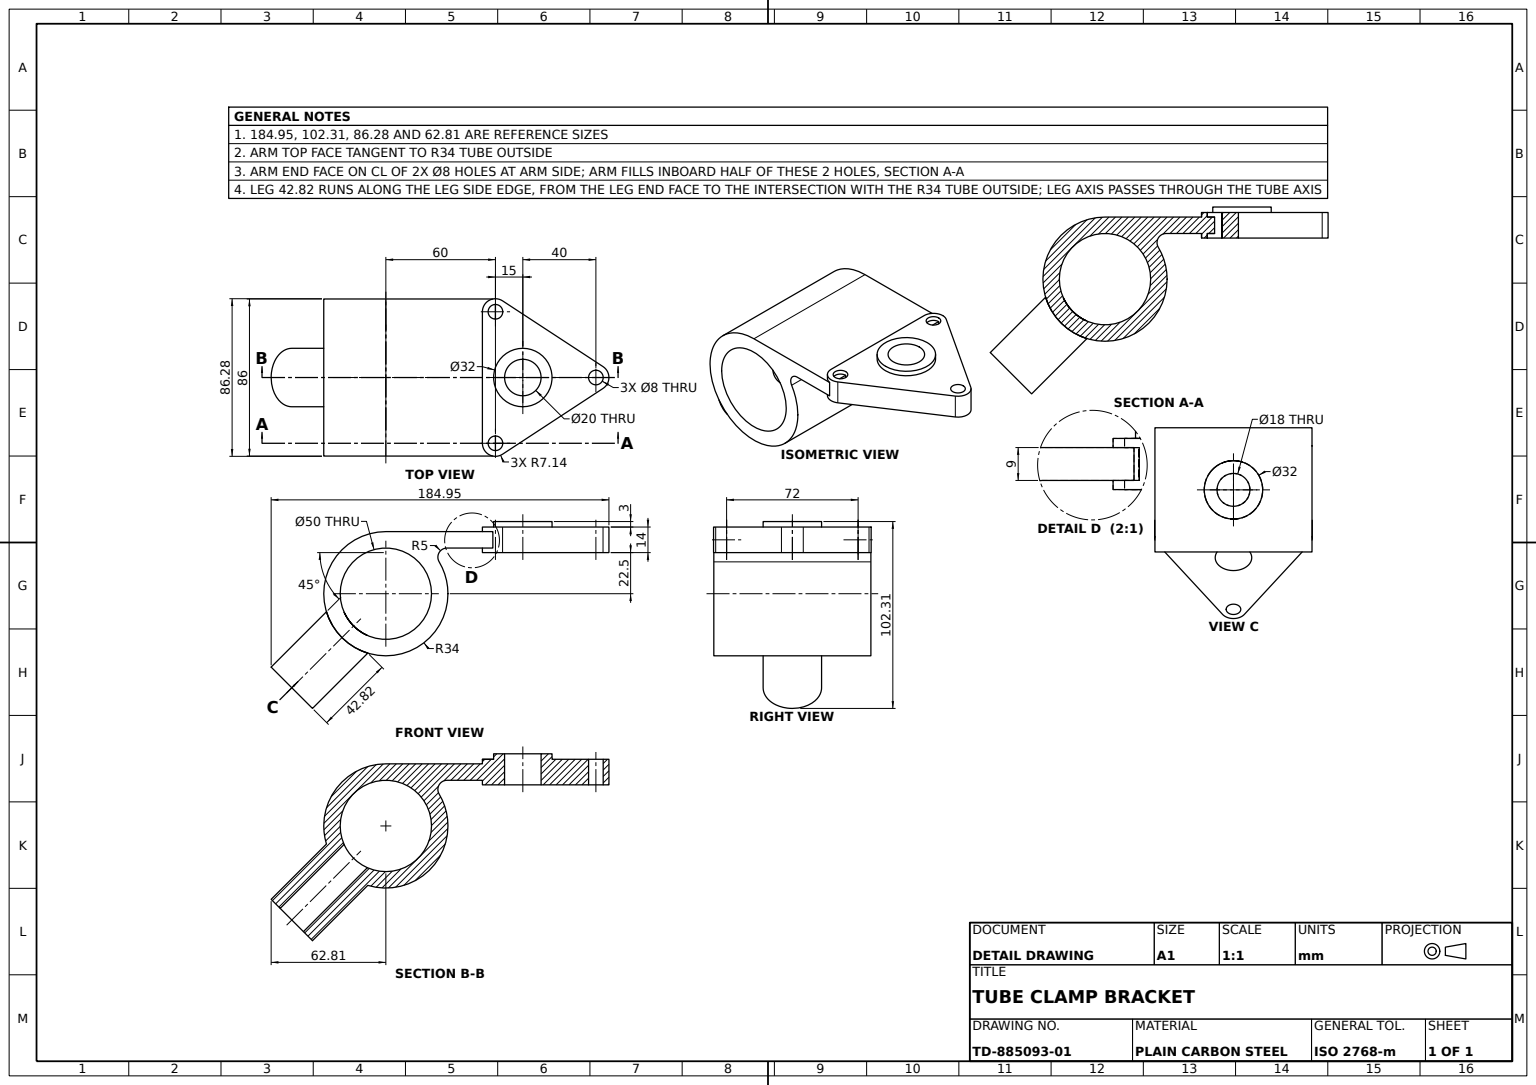
from build123d import *

# Parameters (mm, degrees)
RING_HUB_PROFILE_R       = 25
RING_HUB_DEPTH           = 43
FLANGE_PROFILE_3_HOLES_R = 4
TRIANGULAR_FLANGE_DEPTH  = 7
BOSS_BORE_PROFILE_R      = 10
BOSS_BORE_DEPTH          = 13
FLANGE_START             = 3
FLANGE_BOSS_PROFILE_R    = 16
FLANGE_BOSS_PROFILE_R_2  = 10
FLANGE_BOSS_32_DEPTH     = 3
HUB_SLIT_PROFILE_R       = 9
HUB_SLIT_CUT_DEPTH       = 67.5


with BuildPart() as part:
    # Ring Hub Profile → Ring Hub (new, symmetric)
    with BuildSketch(Plane.XY):
        with BuildLine():
            Line((0, 34), (60, 34))
            Line((60, 34), (60, 25))
            Line((60, 25), (33.481338086, 25))
            ThreePointArc((33.481338086, 25), (29.132745622, 22.467740584), (29.188858844, 17.435897436))
            ThreePointArc((29.188858844, 17.435897436), (-16.780635971, -29.570428749), (0, 34))
        make_face()
        Circle(RING_HUB_PROFILE_R, mode=Mode.SUBTRACT)
    extrude(amount=RING_HUB_DEPTH, both=True)

    # Flange Profile 3 Holes → Triangular Flange (add, symmetric)
    with BuildSketch(Plane(origin=(0, 29.5, 0), x_dir=(1, 0, 0), z_dir=(0, 1, 0))):
        with BuildLine():
            Line((63.910945409, 41.975055486), (118.910945409, 5.975055486))
            ThreePointArc((118.910945409, 5.975055486), (122.141203123, 0), (118.910945409, -5.975055486))
            Line((118.910945409, -5.975055486), (63.910945409, -41.975055486))
            ThreePointArc((63.910945409, -41.975055486), (56.603831094, -42.281943872), (52.858796877, -36))
            Line((52.858796877, -36), (52.858796877, 36))
            ThreePointArc((52.858796877, 36), (56.603831094, 42.281943872), (63.910945409, 41.975055486))
        make_face()
        with Locations(Location((60, 36, 0), (0, 0, 270))):
            Circle(FLANGE_PROFILE_3_HOLES_R, mode=Mode.SUBTRACT)
        with Locations(Location((60, -36, 0), (0, 0, 270))):
            Circle(FLANGE_PROFILE_3_HOLES_R, mode=Mode.SUBTRACT)
        with Locations(Location((115, 0, 0), (0, 0, 270))):
            Circle(FLANGE_PROFILE_3_HOLES_R, mode=Mode.SUBTRACT)
    extrude(amount=TRIANGULAR_FLANGE_DEPTH, both=True)

    # Boss Bore Profile → Boss Bore (cut, symmetric)
    with BuildSketch(Plane(origin=(0, 29.5, 0), x_dir=(1, 0, 0), z_dir=(0, 1, 0))):
        with Locations(Location((75, 0, 0), (0, 0, 270))):
            Circle(BOSS_BORE_PROFILE_R)
    extrude(amount=BOSS_BORE_DEPTH, both=True, mode=Mode.SUBTRACT)

    # Flange Boss Profile → Flange Boss Ø32 (add)
    with BuildSketch(Plane(origin=(0, 36.5, 0), x_dir=(1, 0, 0), z_dir=(0, 1, 0)).offset(FLANGE_START)):
        with Locations(Location((75, 0, 0), (0, 0, 270))):
            Circle(FLANGE_BOSS_PROFILE_R)
        with Locations(Location((75, 0, 0), (0, 0, 270))):
            Circle(FLANGE_BOSS_PROFILE_R_2, mode=Mode.SUBTRACT)
    extrude(amount=-FLANGE_BOSS_32_DEPTH)

    # Hub Revolve Profile → Hub Revolved Feature (revolve)
    with BuildSketch(Plane.XY):
        with BuildLine():
            Line((-32.526911935, -9.899494937), (-62.805081277, -40.177664279))
            Line((-62.805081277, -40.177664279), (-57.855333809, -45.127411748))
            Line((-57.855333809, -45.127411748), (-29.548007269, -16.820085208))
            ThreePointArc((-29.548007269, -16.820085208), (-31.229754097, -13.442561476), (-32.526911935, -9.899494937))
        make_face()
    revolve(axis=Axis((0, 0, 0), (-0.7071067811865461, -0.707106781186549, 0)))

    # Hub Slit Profile → Hub Slit Cut (cut, symmetric)
    with BuildSketch(Plane(origin=(-51.491372778, -51.491372778, 0), x_dir=(0, 0, 1), z_dir=(-0.7071067811865462, -0.7071067811865489, 0))):
        with Locations(Location((0, 0, 0), (0, 0, 90))):
            Circle(HUB_SLIT_PROFILE_R)
    extrude(amount=HUB_SLIT_CUT_DEPTH, both=True, mode=Mode.SUBTRACT)


solid = part.part
